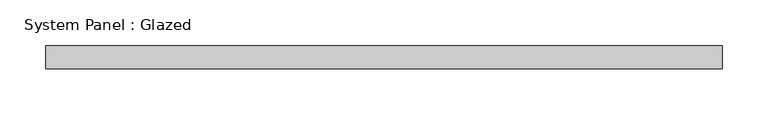
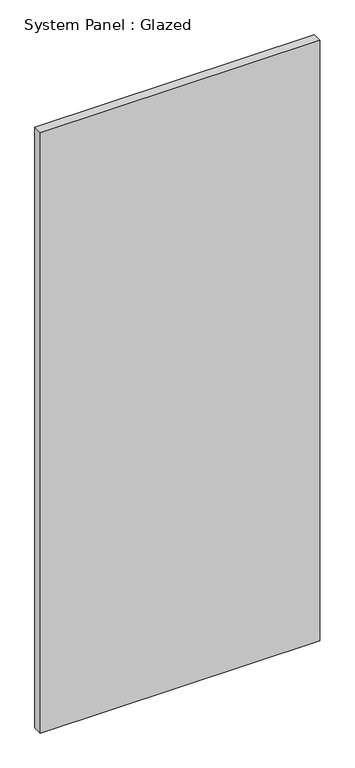
"""IFC4 building model written with IfcOpenShell, lengths in millimetres: plate geometry, System Panel : Glazed."""

from ifc_helpers import new_model, si_unit, origin, origin_with_axes, place, context, project, spatial, polyline, outline, extrude, source, transform, mapped, element, save


def system_panel_glazed_137e22aa(model_context):
    return source(origin(), model_context, "Body", "SweptSolid", [
        extrude(outline(polyline([(370.4021, 19.05), (-370.4021, 19.05), (-370.4021, 44.45), (370.4021, 44.45), (370.4021, 19.05)])), origin_with_axes(), (0.0, 0.0, 1.0), 1682.75),
    ])


if __name__ == "__main__":
    model = new_model("IFC4")
    model_context = context("Model", 3, world=origin())
    ifc_project = project(units=[si_unit("LENGTHUNIT", "METRE", prefix="MILLI")], contexts=[model_context])
    site = spatial("IfcSite", under=ifc_project)
    building = spatial("IfcBuilding", under=site)
    placement = place(None, origin())
    system_panel_glazed_shape = system_panel_glazed_137e22aa(model_context)
    element("IfcPlate", 1, ObjectType="System Panel : Glazed", at=placement, inside=building, context=model_context, shape_type="MappedRepresentation", body=[
        mapped(system_panel_glazed_shape, transform((0.0, 0.0, 0.0), x_axis=(1.0, 0.0, 0.0), y_axis=(0.0, 1.0, 0.0), z_axis=(0.0, 0.0, 1.0))),
    ])
    save(model, "model.ifc")

# Revit data of these elements
# Type "System Panel : Glazed"
#   Construction Type Id = "GSP4R"
#   Analytic Construction = "1/8 in Pilkington single glazing"
#   Visual Light Transmittance = 0.9
#   Solar Heat Gain Coefficient = 0.86
#   Heat Transfer Coefficient (U) = 1.18115 BTU/(h·ft²·°F)
#   Define Thermal Properties by = 1
# Element 1 (IfcPlate, "System Panel : Glazed")
#   Materials on its faces: "Glass"
# Materials
#   "Glass": class "Glass", colour RGB 0 128 192, transparency 0.75, Description = "Soda Lime Glass", Cost = 0
